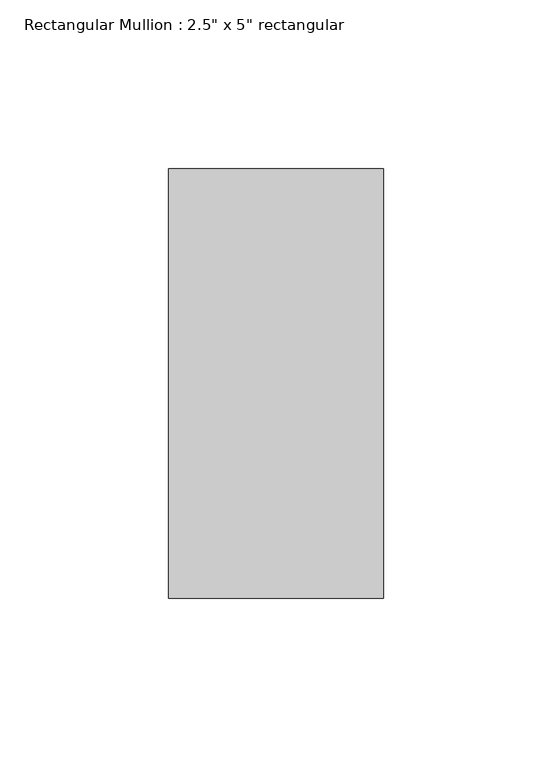
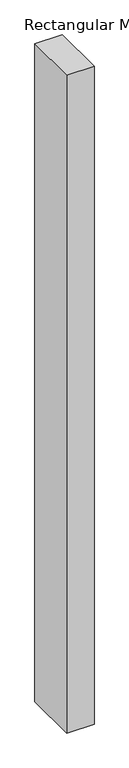
"""IFC4 building model written with IfcOpenShell, lengths in millimetres: member geometry."""

from ifc_helpers import new_model, si_unit, frame, origin, place, context, project, spatial, polyline, outline, extrude, source, transform, mapped, element, save


def member_1afc5165(model_context):
    return source(origin(), model_context, "Body", "SweptSolid", [
        extrude(outline(polyline([(31.75, 63.5), (31.75, -63.5), (-31.75, -63.5), (-31.75, 63.5), (31.75, 63.5)])), frame((0.0, 0.0, -1609.522501), z_axis=(0.0, 0.0, 1.0), x_axis=(1.0, 0.0, 0.0)), (0.0, 0.0, 1.0), 1609.522501),
    ])


if __name__ == "__main__":
    model = new_model("IFC4")
    model_context = context("Model", 3, world=origin())
    ifc_project = project(units=[si_unit("LENGTHUNIT", "METRE", prefix="MILLI")], contexts=[model_context])
    site = spatial("IfcSite", under=ifc_project)
    building = spatial("IfcBuilding", under=site)
    placement = place(None, origin())
    member_shape = member_1afc5165(model_context)
    element("IfcMember", 1, ObjectType="Rectangular Mullion : 2.5\" x 5\" rectangular", at=placement, inside=building, context=model_context, shape_type="MappedRepresentation", body=[
        mapped(member_shape, transform((0.0, 0.0, 0.0), x_axis=(1.0, 0.0, 0.0), y_axis=(0.0, 1.0, 0.0), z_axis=(0.0, 0.0, 1.0))),
    ])
    save(model, "model.ifc")

# Revit data of these elements
# Type "Rectangular Mullion : 2.5\" x 5\" rectangular"
#   built-in parameter 1007304 = 0.416667 (stored number, unit not read)
#   built-in parameter 1007301 = 0.104167 (stored number, unit not read)
#   built-in parameter 1007300 = 0.104167 (stored number, unit not read)
# Element 1 (IfcMember, "Rectangular Mullion : 2.5\" x 5\" rectangular")
#   Materials on its faces: "Aluminum"
# Materials
#   "Aluminum": class "Metal", colour RGB 247 247 247, transparency 0, Description = "Aluminum 6061", Cost = 0
